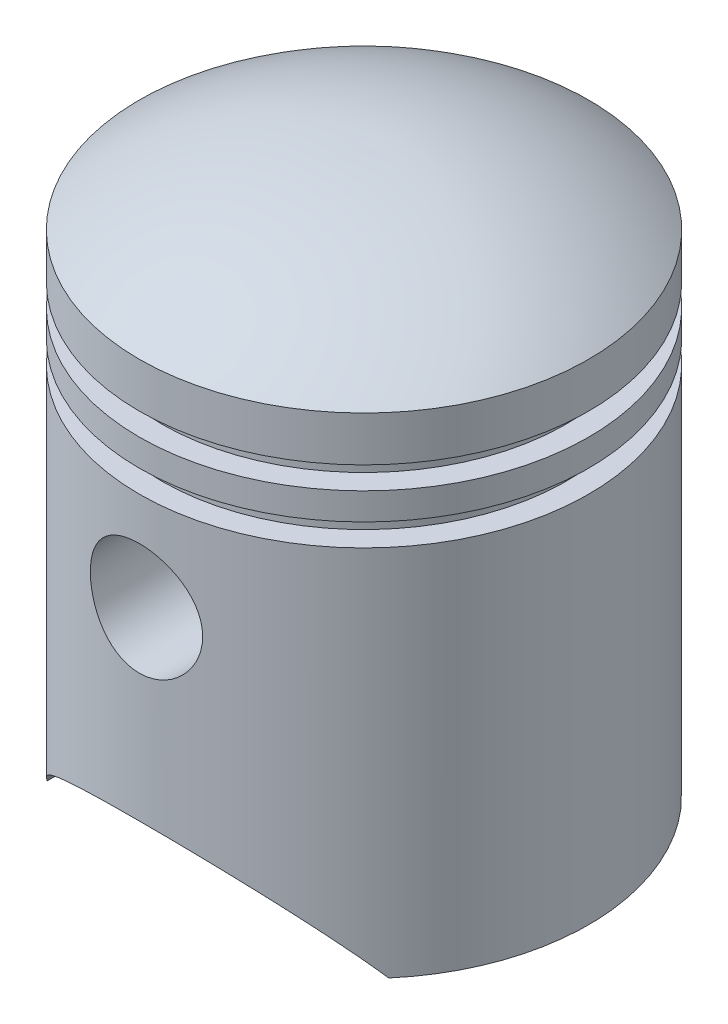
from build123d import *

# Parameters (mm, degrees)
SKIRT_RELIEF_CUT_DEPTH      = 72.817566835
SKIRT_RELIEF_CUT_DEPTH_BACK = 72.817566835
SKIRT_RELIEF_SKETCH_R       = 6.25
PIN_BOSS_REACH              = 85.818
PIN_BOSS_END_RADIUS         = 23
PIN_START                   = 12
PIN_BOSS_SKETCH_R           = 7.25
PIN_BOSS_SKETCH_R_2         = 6.25


with BuildPart() as part:
    # Piston Profile Sketch → Piston Body with Ring Grooves (revolve)
    with BuildSketch(Plane.XY, mode=Mode.PRIVATE) as piston_body_with_ring_grooves_sk:
        with BuildLine():
            Line((25, 0), (25, 41.5))
            Line((25, 41.5), (22.5, 41.5))
            Line((22.5, 41.5), (22.5, 44))
            Line((22.5, 44), (25, 44))
            Line((25, 44), (25, 47))
            Line((25, 47), (22.5, 47))
            Line((22.5, 47), (22.5, 49.5))
            Line((22.5, 49.5), (25, 49.5))
            Line((25, 49.5), (25, 54.5))
            ThreePointArc((25, 54.5), (13.174901691, 60.609067785), (0, 62.5))
            Line((0, 62.5), (0, 60.49936285))
            ThreePointArc((0, 60.49936285), (12.069492637, 58.859165445), (23, 53.484511145))
            Line((23, 53.484511145), (23, 51.5))
            Line((23, 51.5), (20.5, 51.5))
            Line((20.5, 51.5), (20.5, 45.5))
            Line((20.5, 45.5), (20.5, 39.5))
            Line((20.5, 39.5), (23, 39.5))
            Line((23, 39.5), (23, 0))
            Line((23, 0), (25, 0))
        make_face()
    revolve(piston_body_with_ring_grooves_sk.sketch.rotate(Axis((0, 62.5, 0), (0, -1, 0)), 90), axis=Axis((0, 62.5, 0), (0, -1, 0)))

    # Skirt Relief Sketch → Skirt Relief Cut (cut, two sides: drawn at the far end of the back side and taken through both)
    with BuildSketch(Plane.XY.offset(-SKIRT_RELIEF_CUT_DEPTH_BACK)):
        with Locations((0, 30.5)):
            Circle(SKIRT_RELIEF_SKETCH_R)
        with BuildLine():
            Line((-19, 0), (19, 0))
            ThreePointArc((19, 0), (0, 10), (-19, 0))
        make_face()
    extrude(amount=SKIRT_RELIEF_CUT_DEPTH + SKIRT_RELIEF_CUT_DEPTH_BACK, mode=Mode.SUBTRACT)

    # Pin Boss: up to this cylinder (the profile starts inside it)
    pin_boss_end = Plane(origin=(0, 23.455061, 0), z_dir=(0, 1, 0)) * Cylinder(PIN_BOSS_END_RADIUS, 218.636, mode=Mode.PRIVATE)
    # Pin Boss Sketch → Pin Boss (add, up to the surface)
    with BuildSketch(Plane.XY.offset(PIN_START), mode=Mode.PRIVATE) as pin_boss_sk1:
        with Locations(Location((0, 30.5, 0), (0, 0, 90))):
            Circle(PIN_BOSS_SKETCH_R)
        with Locations((0, 30.5)):
            Circle(PIN_BOSS_SKETCH_R_2, mode=Mode.SUBTRACT)
    pin_boss_tool1 = extrude(pin_boss_sk1.sketch, amount=PIN_BOSS_REACH, mode=Mode.PRIVATE) & pin_boss_end
    pin_boss = pin_boss_tool1.solids().sort_by_distance((0, 23.455061, 12))[0]
    add(pin_boss)

    # Pin Boss Mirror: Pin Boss across plane
    add(pin_boss.mirror(Plane.XY))


solid = part.part
